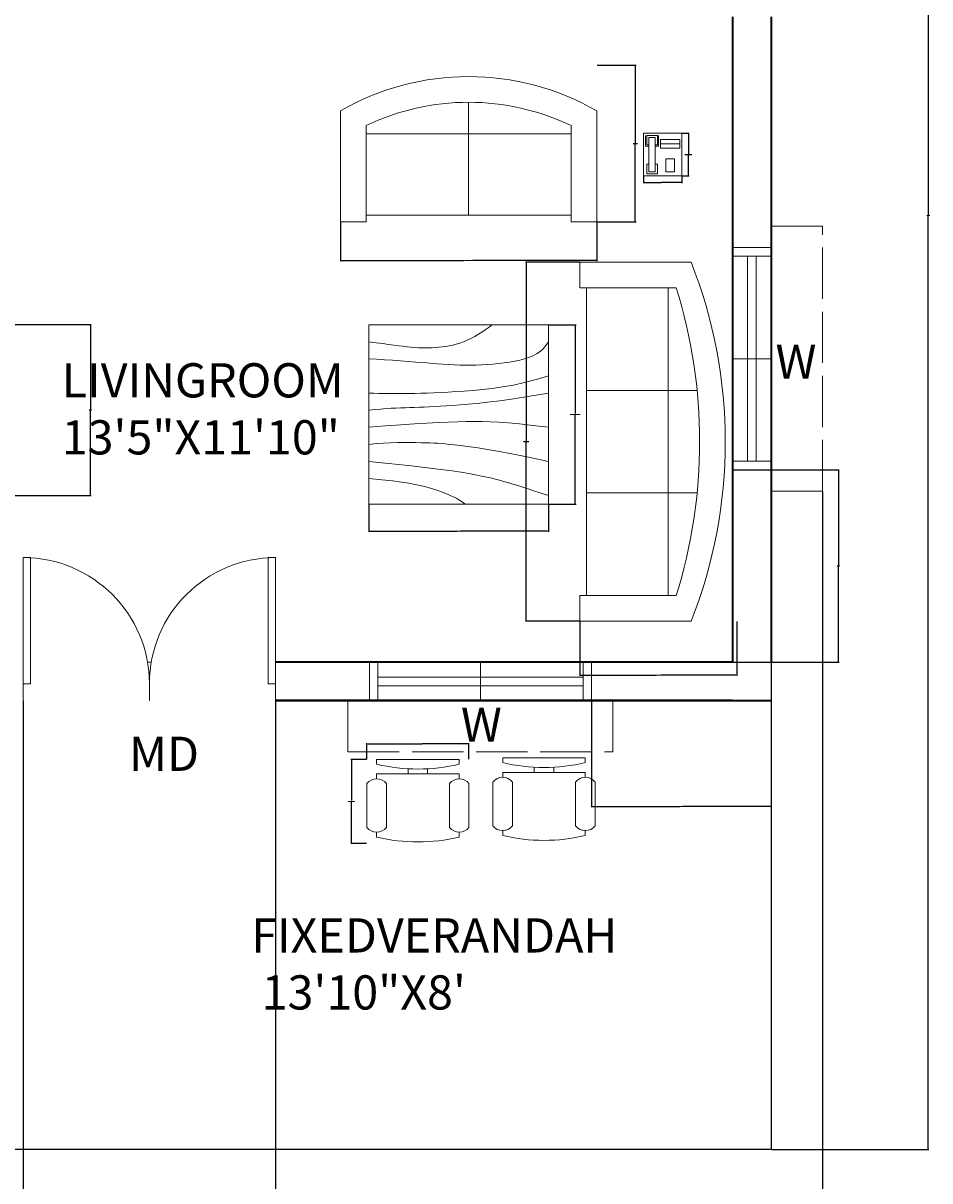
# Model space of a CAD drawing. Units: inches. Extents: x -35 to 832, y -515 to 219.
# Tile 4 of 7: x 179 to 391, y -262 to 9. Entities that reach past the tile are written whole.
import ezdxf

# ---------------------------------------------------------------- set-up
doc = ezdxf.new("R2010")
doc.units = ezdxf.units.IN
doc.header["$MEASUREMENT"] = 0
doc.linetypes.add('ACAD_ISO02W100', pattern=[15, 12, -3])
for name, color, linetype, lineweight in [('A-ANNO-TEXT', 7, 'Continuous', 18), ('A-AREA-IDEN', 7, 'Continuous', 18), ('A-DOOR', 4, 'Continuous', 18), ('A-EQPM', 8, 'Continuous', 18), ('A-FLOR', 7, 'Continuous', 25), ('A-FURN', 8, 'Continuous', 18), ('A-GLAZ', 2, 'Continuous', 18), ('A-GLAZ-OVHD', 2, 'ACAD_ISO02W100', 13), ('A-WALL', 10, 'Continuous', 35), ('S-ANNO-DIMS', 2, 'Continuous', 18)]:
    doc.layers.add(name, color=color, linetype=linetype, lineweight=lineweight)
doc.styles.get("Standard").update_dxf_attribs({"font": 'arial.ttf'})
doc.dimstyles.get("Standard").update_dxf_attribs({"dimtxt": 0.18, "dimasz": 0.18, "dimexe": 0.18, "dimexo": 0.0625, "dimgap": 0.09, "dimtad": 0, "dimtih": 1, "dimtoh": 1, "dimdec": 1, "dimzin": 0, "dimdsep": 46, "dimlunit": 4, "dimtxsty": 'Standard', "dimcen": 0.09, "dimclrd": 211, "dimclre": 4, "dimclrt": 3, "dimadec": 0, "dimazin": 0, "dimtfac": 0.5, "dimtdec": 1, "dimtofl": 0, "dimtmove": 0, "dimatfit": 3, "dimfxl": 1, "dimtfill": 2, "dimtfillclr": 61, "dimtolj": 1, "dimtzin": 0, "dimarcsym": 0})

# ---------------------------------------------------------------- blocks, each defined once
blk = doc.blocks.new('Chair - Desk')
for p, q in [((-8.5, 0), (-8.5, -1)), ((-8.5, 0), (8.5, 0)), ((8.5, 0), (8.5, -1)), ((-2, -3), (-2, -1.9355)), ((2, -1.9576), (2, -3)), ((-8.5, -3), (-8.5, -4)), ((-8.5, -3), (8.5, -3)), ((8.5, -3), (8.5, -4)), ((-10.5, -5), (-10.5, -14)), ((-6.5, -14), (-6.5, -5)), ((6.5, -5), (6.5, -14)), ((10.5, -14), (10.5, -5)), ((-8.5, -15), (-8.5, -16)), ((8.5, -15), (8.5, -16))]:
    blk.add_line(p, q)
for centre, radius, start, end in [((0, 34.625), 36.625, 256.5803, 283.4197), ((-8.5, -6.5), 2.5, 36.8699, 143.1301), ((8.5, -6.5), 2.5, 36.8699, 143.1301), ((-8.5, -12.5), 2.5, 216.8699, 323.1301), ((8.5, -12.5), 2.5, 216.8699, 323.1301), ((0, 19.625), 36.625, 256.5803, 283.4197)]:
    blk.add_arc(centre, radius, start, end)
blk = doc.blocks.new('Table - Square Woodgrain 42 x 42 in.')
blk.add_line((0, -42), (42, -42))
for points in [[(0, -4), (1.704, -4.2172), (3.2358, -4.4188), (4.615, -4.604), (5.8615, -4.7721), (6.9951, -4.9224), (8.0357, -5.0541), (9.0031, -5.1667), (9.9171, -5.2594), (10.7951, -5.3316), (11.6445, -5.3836), (12.4702, -5.4157), (13.277, -5.4283), (14.0698, -5.4217), (14.8535, -5.3964), (15.6331, -5.3526), (16.4133, -5.2908), (17.1986, -5.2103), (17.9913, -5.1062), (18.793, -4.9727), (19.6056, -4.8038), (20.4307, -4.5937), (21.2701, -4.3365), (22.1256, -4.0262), (22.9989, -3.6571), (23.888, -3.2272), (24.7756, -2.7516), (25.6408, -2.2491), (26.4624, -1.7387), (27.2195, -1.2395), (27.891, -0.7703), (28.456, -0.3501), (28.8934, 0.002)], [(0, -42), (0, 0), (42, 0), (42, -42)], [(0, -8), (1.8203, -8.1001), (3.6741, -8.2149), (5.5411, -8.3408), (7.4011, -8.4741), (9.2339, -8.6112), (11.0193, -8.7484), (12.7371, -8.8821), (14.3671, -9.0086), (15.8954, -9.1246), (17.3337, -9.2278), (18.6997, -9.3159), (20.0116, -9.387), (21.2871, -9.4389), (22.5442, -9.4696), (23.8008, -9.477), (25.0749, -9.459), (26.3791, -9.4137), (27.7049, -9.3403), (29.0383, -9.2382), (30.3655, -9.1068), (31.6728, -8.9455), (32.9461, -8.7535), (34.1717, -8.5304), (35.3358, -8.2756), (36.4268, -7.9863), (37.443, -7.6521), (38.3849, -7.2603), (39.253, -6.7986), (40.048, -6.2542), (40.7705, -5.6147), (41.421, -4.8674), (42, -4)], [(42, -12), (39.1784, -12.8621), (36.4519, -13.5654), (33.8246, -14.1294), (31.3004, -14.5731), (28.8832, -14.9161), (26.577, -15.1775), (24.3858, -15.3768), (22.3136, -15.5332), (20.3622, -15.6632), (18.5254, -15.7718), (16.7947, -15.8612), (15.1618, -15.9338), (13.6183, -15.9916), (12.1558, -16.0369), (10.7659, -16.0718), (9.4403, -16.0987), (8.1703, -16.1191), (6.9461, -16.1325), (5.7577, -16.1377), (4.595, -16.1335), (3.4479, -16.1188), (2.3064, -16.0924), (1.1604, -16.0532), (0, -16)], [(42, -16), (37.6529, -16.7365), (33.8802, -17.329), (30.6179, -17.7961), (27.8015, -18.1561), (25.3668, -18.4275), (23.2497, -18.6288), (21.3859, -18.7785), (19.7111, -18.8949), (18.1693, -18.9939), (16.7375, -19.0795), (15.401, -19.1534), (14.1449, -19.217), (12.9544, -19.2717), (11.8148, -19.3191), (10.7113, -19.3606), (9.6291, -19.3976), (8.5534, -19.4323), (7.47, -19.4689), (6.3643, -19.5122), (5.222, -19.5672), (4.0288, -19.6386), (2.7703, -19.7313), (1.4321, -19.8501), (0, -20)], [(0, -24), (3.9243, -23.6805), (7.4766, -23.4138), (10.6891, -23.1954), (13.5943, -23.0205), (16.2247, -22.8847), (18.6125, -22.7832), (20.7903, -22.7116), (22.7903, -22.6651), (24.6563, -22.642), (26.4764, -22.6507), (28.35, -22.7024), (30.3766, -22.8084), (32.6555, -22.98), (35.2861, -23.2283), (38.3678, -23.5645), (42, -24)], [(42, -32), (37.392, -31.017), (33.4585, -30.2231), (30.1291, -29.5949), (27.3334, -29.109), (25.0009, -28.742), (23.0612, -28.4707), (21.4439, -28.2716), (20.0786, -28.1215), (18.8998, -28.0002), (17.8609, -27.9014), (16.9206, -27.8219), (16.0371, -27.7588), (15.1691, -27.709), (14.2748, -27.6693), (13.3128, -27.6368), (12.2415, -27.6083), (11.0295, -27.5824), (9.6867, -27.5643), (8.233, -27.5608), (6.6884, -27.5787), (5.0728, -27.6248), (3.4062, -27.7058), (1.7086, -27.8286), (0, -28)], [(0, -32), (5.4026, -32.5358), (9.9494, -33.019), (13.7424, -33.4553), (16.8834, -33.8505), (19.4743, -34.2106), (21.6171, -34.5413), (23.4136, -34.8486), (24.9657, -35.1382), (26.3614, -35.4156), (27.6332, -35.6841), (28.7995, -35.9467), (29.8788, -36.2064), (30.8897, -36.4661), (31.8507, -36.7288), (32.7802, -36.9973), (33.6968, -37.2747), (34.6175, -37.5635), (35.5531, -37.8651), (36.5128, -38.1805), (37.506, -38.5108), (38.5421, -38.8568), (39.6302, -39.2197), (40.7797, -39.6004), (42, -40)], [(0, -36), (3.0098, -36.2857), (5.5354, -36.5643), (7.6368, -36.8359), (9.374, -37.1009), (10.807, -37.3597), (11.9957, -37.6126), (13.0002, -37.8599), (13.8804, -38.102), (14.6874, -38.3393), (15.4365, -38.5729), (16.1338, -38.8041), (16.7858, -39.0341), (17.3987, -39.264), (17.9787, -39.4952), (18.5322, -39.7288), (19.0655, -39.9662), (19.5832, -40.2081), (20.0842, -40.4544), (20.5657, -40.7046), (21.0249, -40.9581), (21.459, -41.2144), (21.8653, -41.4731), (22.2409, -41.7335), (22.5831, -41.9951)]]:
    blk.add_lwpolyline(points)
blk = doc.blocks.new('Sofa - Roundback 7 ft.')
for p, q in [((-12.00002, -32.4421), (-12.00003, -6.5971)), ((11.99997, -32.4421), (11.99998, -6.5971)), ((-36.000027, -34), (-36.000027, -11.4696)), ((-35.999844, -13.3819), (35.9998, -13.3819)), ((35.99998, -34), (35.99998, -11.4696)), ((-36.000027, -32.4421), (35.99998, -32.4421))]:
    blk.add_line(p, q)
for points in [[(-36.000027, -34), (-42.000027, -34), (-42.000027, -8)], [(41.99998, -8), (41.99998, -34), (35.99998, -34)]]:
    blk.add_lwpolyline(points)
for centre, radius, start, end in [((0, -114.25), 114.25, 68.43141, 111.5686), ((-0.00001, -127.1968), 121.1968, 72.72033, 107.2797)]:
    blk.add_arc(centre, radius, start, end)
blk = doc.blocks.new('Sofa - Roundback Loveseat 5 ft.')
for p, q in [((0, -32.44198), (0, -5.99998)), ((-24, -33.99998), (-24, -11.46958)), ((-23.9998, -13.38178), (23.99986, -13.38178)), ((24.00004, -33.99998), (24.00004, -11.46958)), ((-24, -32.44198), (24.00004, -32.44198))]:
    blk.add_line(p, q)
for points in [[(-24, -33.99998), (-30, -33.99998), (-30, -7.99998)], [(30.00004, -7.99998), (30.00004, -33.99998), (24.00004, -33.99998)]]:
    blk.add_lwpolyline(points)
for centre, radius, start, end in [((0, -60.24998), 60.24998, 60.13715, 119.8628), ((0, -61.38438), 55.38444, 64.32083, 115.6792)]:
    blk.add_arc(centre, radius, start, end)
blk = doc.blocks.new('Phone - Desk')
for p, q in [((-4.5, -5), (-4.5, 5)), ((-4.5, 5), (4.5, 5)), ((-4, 4.5), (-4, 2)), ((-3.75, 4.5), (-3.75, 2.25)), ((-1.25, 4.5), (-3.75, 4.5)), ((-3.25, 4), (-3.25, -4)), ((-3.25, 4), (-1.75, 4)), ((-1.75, -4), (-1.75, 4)), ((-1.25, 2.25), (-1.25, 4.5)), ((-1, 2), (-1, 4.5)), ((4, 3.5), (-0.5, 3.5)), ((-0.5, 3.5), (-0.5, 1.5)), ((4, 1.5), (4, 3.5)), ((4.5, 5), (4.5, -5)), ((-4, 2), (-3.25, 2)), ((-3.75, 2.25), (-3.25, 2.25)), ((-1.75, 2.25), (-1.25, 2.25)), ((-1.75, 2), (-1, 2)), ((-0.5, 2.5), (4, 2.5)), ((-0.5, 1.5), (4, 1.5)), ((-3.75, -2.25), (-3.25, -2.25)), ((-3.75, -4.5), (-3.75, -2.25)), ((-1.75, -2.25), (-1.25, -2.25)), ((-1.25, -2.25), (-1.25, -4.5)), ((2.75, -1), (0.75, -1)), ((0.75, -1), (0.75, -4)), ((2.75, -4), (2.75, -1)), ((4.5, -5), (-4.5, -5)), ((-1.25, -4.5), (-3.75, -4.5)), ((-3.25, -4), (-1.75, -4)), ((0.75, -4), (2.75, -4))]:
    blk.add_line(p, q)
blk = doc.blocks.new('*U4')
for p, q in [((0, 0), (0, -100)), ((750, 0), (750, -100))]:
    blk.add_line(p, q)
blk.add_lwpolyline([(0, 0), (0, 750), (43.75, 750), (43.75, 0)], close=True)
blk.add_arc((0, 0), 750, 0, 90)
blk = doc.blocks.new('WIN-48')
for p, q in [((0, 9), (0, 0)), ((2, 9), (2, 0)), ((26, 9), (26, 0)), ((50, 9), (50, 0)), ((52, 9), (52, 0)), ((2, 5.5), (50, 5.5)), ((2, 3.5), (50, 3.5))]:
    blk.add_line(p, q)
blk = doc.blocks.new('WIN-48-HOOD')
for p, q in [((5, 12), (0, 12)), ((0, 12), (0, 0)), ((57, 12), (62, 12)), ((62, 12), (62, 0)), ((0, 0), (62, 0))]:
    blk.add_line(p, q)
blk = doc.blocks.new('*D71')
at = {"layer": 'Defpoints', "color": 0, "transparency": 16777216}
for p in [(283.1, -160.09), (259.23, -163.68), (283.1, -163.68)]:
    blk.add_point(p, dxfattribs=at)
at = {"layer": 'S-ANNO-DIMS', "color": 4, "lineweight": -2, "transparency": 16777216}
for p, q in [((259.23, -163.61), (259.23, -159.91)), ((283.1, -163.61), (283.1, -159.91))]:
    blk.add_line(p, q, dxfattribs=at)
at = {"layer": 'S-ANNO-DIMS', "color": 211, "lineweight": -2, "transparency": 16777216}
for p, q in [((259.41, -160.09), (270.1, -160.09)), ((282.92, -160.09), (272.23, -160.09))]:
    blk.add_line(p, q, dxfattribs=at)
at = {"layer": 'S-ANNO-DIMS', "color": 211, "transparency": 16777216}
for points in [[(259.41, -160.06), (259.41, -160.12), (259.23, -160.09)], [(282.92, -160.06), (282.92, -160.12), (283.1, -160.09)]]:
    blk.add_solid(points, dxfattribs=at)
at = {"layer": 'S-ANNO-DIMS', "color": 3, "transparency": 16777216, "insert": (271.17, -160.09), "char_height": 0.18, "attachment_point": 5, "bg_fill": 1, "box_fill_scale": 1.25, "bg_fill_color": 61, "bg_fill_transparency": 0}
blk.add_mtext('\\A1;CHAIR 2\'-0" TYP.', dxfattribs=at)
blk = doc.blocks.new('*D72')
at = {"layer": 'Defpoints', "color": 0, "transparency": 16777216}
for p in [(255.65, -163.68), (259.23, -163.68), (259.23, -183.38)]:
    blk.add_point(p, dxfattribs=at)
at = {"layer": 'S-ANNO-DIMS', "color": 4, "lineweight": -2, "transparency": 16777216}
for p, q in [((259.17, -163.68), (255.47, -163.68)), ((259.17, -183.38), (255.47, -183.38))]:
    blk.add_line(p, q, dxfattribs=at)
at = {"layer": 'S-ANNO-DIMS', "color": 211, "lineweight": -2, "transparency": 16777216}
for p, q in [((255.65, -163.86), (255.65, -173.34)), ((255.65, -183.2), (255.65, -173.71))]:
    blk.add_line(p, q, dxfattribs=at)
at = {"layer": 'S-ANNO-DIMS', "color": 211, "transparency": 16777216}
for points in [[(255.62, -163.86), (255.68, -163.86), (255.65, -163.68)], [(255.62, -183.2), (255.68, -183.2), (255.65, -183.38)]]:
    blk.add_solid(points, dxfattribs=at)
at = {"layer": 'S-ANNO-DIMS', "color": 3, "transparency": 16777216, "insert": (255.65, -173.53), "char_height": 0.18, "attachment_point": 5, "bg_fill": 1, "box_fill_scale": 1.25, "bg_fill_color": 61, "bg_fill_transparency": 0}
blk.add_mtext('\\A1;1\'-7 1/2" TYP.', dxfattribs=at)
blk = doc.blocks.new('*D95')
at = {"layer": 'Defpoints', "color": 0, "transparency": 16777216}
for p in [(301.68, -61.99), (307.98, -61.99), (301.68, -103.99)]:
    blk.add_point(p, dxfattribs=at)
at = {"layer": 'S-ANNO-DIMS', "color": 4, "lineweight": -2, "transparency": 16777216}
for p, q in [((301.74, -61.99), (308.16, -61.99)), ((301.74, -103.99), (308.16, -103.99))]:
    blk.add_line(p, q, dxfattribs=at)
at = {"layer": 'S-ANNO-DIMS', "color": 211, "lineweight": -2, "transparency": 16777216}
for p, q in [((307.98, -62.17), (307.98, -82.81)), ((307.98, -103.81), (307.98, -83.18))]:
    blk.add_line(p, q, dxfattribs=at)
at = {"layer": 'S-ANNO-DIMS', "color": 211, "transparency": 16777216}
for points in [[(307.95, -62.17), (308.01, -62.17), (307.98, -61.99)], [(307.95, -103.81), (308.01, -103.81), (307.98, -103.99)]]:
    blk.add_solid(points, dxfattribs=at)
at = {"layer": 'S-ANNO-DIMS', "color": 3, "transparency": 16777216, "insert": (307.98, -82.99), "char_height": 0.18, "attachment_point": 5, "bg_fill": 1, "box_fill_scale": 1.25, "bg_fill_color": 61, "bg_fill_transparency": 0}
blk.add_mtext('\\A1;COFFEE TABLE 3\'-6"', dxfattribs=at)
blk = doc.blocks.new('*D96')
at = {"layer": 'Defpoints', "color": 0, "transparency": 16777216}
for p in [(259.68, -103.99), (301.68, -103.99), (301.68, -110.29)]:
    blk.add_point(p, dxfattribs=at)
at = {"layer": 'S-ANNO-DIMS', "color": 4, "lineweight": -2, "transparency": 16777216}
for p, q in [((259.68, -104.06), (259.68, -110.47)), ((301.68, -104.06), (301.68, -110.47))]:
    blk.add_line(p, q, dxfattribs=at)
at = {"layer": 'S-ANNO-DIMS', "color": 211, "lineweight": -2, "transparency": 16777216}
for p, q in [((259.86, -110.29), (280.35, -110.29)), ((301.5, -110.29), (281.01, -110.29))]:
    blk.add_line(p, q, dxfattribs=at)
at = {"layer": 'S-ANNO-DIMS', "color": 211, "transparency": 16777216}
for points in [[(259.86, -110.26), (259.86, -110.32), (259.68, -110.29)], [(301.5, -110.26), (301.5, -110.32), (301.68, -110.29)]]:
    blk.add_solid(points, dxfattribs=at)
at = {"layer": 'S-ANNO-DIMS', "color": 3, "transparency": 16777216, "insert": (280.68, -110.29), "char_height": 0.18, "attachment_point": 5, "bg_fill": 1, "box_fill_scale": 1.25, "bg_fill_color": 61, "bg_fill_transparency": 0}
blk.add_mtext('\\A1;3\'-6"', dxfattribs=at)
blk = doc.blocks.new('*D97')
at = {"layer": 'Defpoints', "color": 0, "transparency": 16777216}
for p in [(309.08, -47.37), (296.48, -131.37), (309.08, -131.37)]:
    blk.add_point(p, dxfattribs=at)
at = {"layer": 'S-ANNO-DIMS', "color": 4, "lineweight": -2, "transparency": 16777216}
for p, q in [((309.02, -47.37), (296.3, -47.37)), ((309.02, -131.37), (296.3, -131.37))]:
    blk.add_line(p, q, dxfattribs=at)
at = {"layer": 'S-ANNO-DIMS', "color": 211, "lineweight": -2, "transparency": 16777216}
for p, q in [((296.48, -47.55), (296.48, -89.19)), ((296.48, -131.19), (296.48, -89.55))]:
    blk.add_line(p, q, dxfattribs=at)
at = {"layer": 'S-ANNO-DIMS', "color": 211, "transparency": 16777216}
for points in [[(296.45, -47.55), (296.51, -47.55), (296.48, -47.37)], [(296.45, -131.19), (296.51, -131.19), (296.48, -131.37)]]:
    blk.add_solid(points, dxfattribs=at)
at = {"layer": 'S-ANNO-DIMS', "color": 3, "transparency": 16777216, "insert": (296.48, -89.37), "char_height": 0.18, "attachment_point": 5, "bg_fill": 1, "box_fill_scale": 1.25, "bg_fill_color": 61, "bg_fill_transparency": 0}
blk.add_mtext('\\A1;SOFA 7\'-0"', dxfattribs=at)
blk = doc.blocks.new('*D98')
at = {"layer": 'Defpoints', "color": 0, "transparency": 16777216}
for p in [(309.08, -131.37), (345.75, -131.37), (345.75, -143.97)]:
    blk.add_point(p, dxfattribs=at)
at = {"layer": 'S-ANNO-DIMS', "color": 4, "lineweight": -2, "transparency": 16777216}
for p, q in [((309.08, -131.43), (309.08, -144.15)), ((345.75, -131.43), (345.75, -144.15))]:
    blk.add_line(p, q, dxfattribs=at)
at = {"layer": 'S-ANNO-DIMS', "color": 211, "lineweight": -2, "transparency": 16777216}
for p, q in [((309.26, -143.97), (326.88, -143.97)), ((345.57, -143.97), (327.96, -143.97))]:
    blk.add_line(p, q, dxfattribs=at)
at = {"layer": 'S-ANNO-DIMS', "color": 211, "transparency": 16777216}
for points in [[(309.26, -143.94), (309.26, -144), (309.08, -143.97)], [(345.57, -143.94), (345.57, -144), (345.75, -143.97)]]:
    blk.add_solid(points, dxfattribs=at)
at = {"layer": 'S-ANNO-DIMS', "color": 3, "transparency": 16777216, "insert": (327.42, -143.97), "char_height": 0.18, "attachment_point": 5, "bg_fill": 1, "box_fill_scale": 1.25, "bg_fill_color": 61, "bg_fill_transparency": 0}
blk.add_mtext('\\A1;3\'-0 1/2"', dxfattribs=at)
blk = doc.blocks.new('*D99')
at = {"layer": 'Defpoints', "color": 0, "transparency": 16777216}
for p in [(253.02, -37.96), (313.02, -37.96), (313.02, -46.96)]:
    blk.add_point(p, dxfattribs=at)
at = {"layer": 'S-ANNO-DIMS', "color": 4, "lineweight": -2, "transparency": 16777216}
for p, q in [((253.02, -38.03), (253.02, -47.14)), ((313.02, -38.03), (313.02, -47.14))]:
    blk.add_line(p, q, dxfattribs=at)
at = {"layer": 'S-ANNO-DIMS', "color": 211, "lineweight": -2, "transparency": 16777216}
for p, q in [((253.2, -46.96), (281.99, -46.96)), ((312.84, -46.96), (284.04, -46.96))]:
    blk.add_line(p, q, dxfattribs=at)
at = {"layer": 'S-ANNO-DIMS', "color": 211, "transparency": 16777216}
for points in [[(253.2, -46.93), (253.2, -46.99), (253.02, -46.96)], [(312.84, -46.93), (312.84, -46.99), (313.02, -46.96)]]:
    blk.add_solid(points, dxfattribs=at)
at = {"layer": 'S-ANNO-DIMS', "color": 3, "transparency": 16777216, "insert": (283.02, -46.96), "char_height": 0.18, "attachment_point": 5, "bg_fill": 1, "box_fill_scale": 1.25, "bg_fill_color": 61, "bg_fill_transparency": 0}
blk.add_mtext('\\A1;LOVESEAT 5\'-0"', dxfattribs=at)
blk = doc.blocks.new('*D100')
at = {"layer": 'Defpoints', "color": 0, "transparency": 16777216}
for p in [(313.02, -1.3), (322.02, -1.3), (313.02, -37.96)]:
    blk.add_point(p, dxfattribs=at)
at = {"layer": 'S-ANNO-DIMS', "color": 4, "lineweight": -2, "transparency": 16777216}
for p, q in [((313.08, -1.3), (322.2, -1.3)), ((313.08, -37.96), (322.2, -37.96))]:
    blk.add_line(p, q, dxfattribs=at)
at = {"layer": 'S-ANNO-DIMS', "color": 211, "lineweight": -2, "transparency": 16777216}
for p, q in [((322.02, -1.48), (322.02, -19.45)), ((322.02, -37.78), (322.02, -19.81))]:
    blk.add_line(p, q, dxfattribs=at)
at = {"layer": 'S-ANNO-DIMS', "color": 211, "transparency": 16777216}
for points in [[(321.99, -1.48), (322.05, -1.48), (322.02, -1.3)], [(321.99, -37.78), (322.05, -37.78), (322.02, -37.96)]]:
    blk.add_solid(points, dxfattribs=at)
at = {"layer": 'S-ANNO-DIMS', "color": 3, "transparency": 16777216, "insert": (322.02, -19.63), "char_height": 0.18, "attachment_point": 5, "bg_fill": 1, "box_fill_scale": 1.25, "bg_fill_color": 61, "bg_fill_transparency": 0}
blk.add_mtext('\\A1;3\'-0 1/2"', dxfattribs=at)
blk = doc.blocks.new('*D101')
at = {"layer": 'Defpoints', "color": 0, "transparency": 16777216}
for p in [(332.94, -17.2), (334.44, -17.2), (332.94, -27.2)]:
    blk.add_point(p, dxfattribs=at)
at = {"layer": 'S-ANNO-DIMS', "color": 4, "lineweight": -2, "transparency": 16777216}
for p, q in [((333, -17.2), (334.62, -17.2)), ((333, -27.2), (334.62, -27.2))]:
    blk.add_line(p, q, dxfattribs=at)
at = {"layer": 'S-ANNO-DIMS', "color": 211, "lineweight": -2, "transparency": 16777216}
for p, q in [((334.44, -17.38), (334.44, -22.02)), ((334.44, -27.02), (334.44, -22.38))]:
    blk.add_line(p, q, dxfattribs=at)
at = {"layer": 'S-ANNO-DIMS', "color": 211, "transparency": 16777216}
for points in [[(334.41, -17.38), (334.47, -17.38), (334.44, -17.2)], [(334.41, -27.02), (334.47, -27.02), (334.44, -27.2)]]:
    blk.add_solid(points, dxfattribs=at)
at = {"layer": 'S-ANNO-DIMS', "color": 3, "transparency": 16777216, "insert": (334.44, -22.2), "char_height": 0.18, "attachment_point": 5, "bg_fill": 1, "box_fill_scale": 1.25, "bg_fill_color": 61, "bg_fill_transparency": 0}
blk.add_mtext('\\A1;PHONE 0\'-10"', dxfattribs=at)
blk = doc.blocks.new('*D102')
at = {"layer": 'Defpoints', "color": 0, "transparency": 16777216}
for p in [(323.94, -27.2), (332.94, -27.2), (332.94, -28.7)]:
    blk.add_point(p, dxfattribs=at)
at = {"layer": 'S-ANNO-DIMS', "color": 4, "lineweight": -2, "transparency": 16777216}
for p, q in [((323.94, -27.26), (323.94, -28.88)), ((332.94, -27.26), (332.94, -28.88))]:
    blk.add_line(p, q, dxfattribs=at)
at = {"layer": 'S-ANNO-DIMS', "color": 211, "lineweight": -2, "transparency": 16777216}
for p, q in [((324.12, -28.7), (328.11, -28.7)), ((332.76, -28.7), (328.77, -28.7))]:
    blk.add_line(p, q, dxfattribs=at)
at = {"layer": 'S-ANNO-DIMS', "color": 211, "transparency": 16777216}
for points in [[(324.12, -28.67), (324.12, -28.73), (323.94, -28.7)], [(332.76, -28.67), (332.76, -28.73), (332.94, -28.7)]]:
    blk.add_solid(points, dxfattribs=at)
at = {"layer": 'S-ANNO-DIMS', "color": 3, "transparency": 16777216, "insert": (328.44, -28.7), "char_height": 0.18, "attachment_point": 5, "bg_fill": 1, "box_fill_scale": 1.25, "bg_fill_color": 61, "bg_fill_transparency": 0}
blk.add_mtext('\\A1;0\'-9"', dxfattribs=at)
blk = doc.blocks.new('*D106')
at = {"layer": 'Defpoints', "color": 0, "transparency": 16777216}
for p in [(353.8, 182.05), (353.8, -254.95), (390.55, -254.95)]:
    blk.add_point(p, dxfattribs=at)
at = {"layer": 'S-ANNO-DIMS', "color": 4, "lineweight": -2, "transparency": 16777216}
for p, q in [((353.86, 182.05), (390.73, 182.05)), ((353.86, -254.95), (390.73, -254.95))]:
    blk.add_line(p, q, dxfattribs=at)
at = {"layer": 'S-ANNO-DIMS', "color": 211, "lineweight": -2, "transparency": 16777216}
for p, q in [((390.55, 181.87), (390.55, -36.27)), ((390.55, -254.77), (390.55, -36.63))]:
    blk.add_line(p, q, dxfattribs=at)
at = {"layer": 'S-ANNO-DIMS', "color": 211, "transparency": 16777216}
for points in [[(390.52, 181.87), (390.58, 181.87), (390.55, 182.05)], [(390.52, -254.77), (390.58, -254.77), (390.55, -254.95)]]:
    blk.add_solid(points, dxfattribs=at)
at = {"layer": 'S-ANNO-DIMS', "color": 3, "transparency": 16777216, "insert": (390.55, -36.45), "char_height": 0.18, "attachment_point": 5, "bg_fill": 1, "box_fill_scale": 1.25, "bg_fill_color": 61, "bg_fill_transparency": 0}
blk.add_mtext('\\A1;36\'-5"', dxfattribs=at)
blk = doc.blocks.new('*D109')
at = {"layer": 'Defpoints', "color": 0, "transparency": 16777216}
for p in [(365.8, -100.95), (-10.2, -143.45), (365.8, -279.7)]:
    blk.add_point(p, dxfattribs=at)
at = {"layer": 'S-ANNO-DIMS', "color": 4, "lineweight": -2, "transparency": 16777216}
for p, q in [((365.8, -101.01), (365.8, -279.88)), ((-10.2, -143.51), (-10.2, -279.88))]:
    blk.add_line(p, q, dxfattribs=at)
at = {"layer": 'S-ANNO-DIMS', "color": 211, "lineweight": -2, "transparency": 16777216}
for p, q in [((-10.02, -279.7), (177.4, -279.7)), ((365.62, -279.7), (178.2, -279.7))]:
    blk.add_line(p, q, dxfattribs=at)
at = {"layer": 'S-ANNO-DIMS', "color": 211, "transparency": 16777216}
for points in [[(-10.02, -279.67), (-10.02, -279.73), (-10.2, -279.7)], [(365.62, -279.67), (365.62, -279.73), (365.8, -279.7)]]:
    blk.add_solid(points, dxfattribs=at)
at = {"layer": 'S-ANNO-DIMS', "color": 3, "transparency": 16777216, "insert": (177.8, -279.7), "char_height": 0.18, "attachment_point": 5, "bg_fill": 1, "box_fill_scale": 1.25, "bg_fill_color": 61, "bg_fill_transparency": 0}
blk.add_mtext('\\A1;31\'-4"', dxfattribs=at)
blk = doc.blocks.new('*D111')
at = {"layer": 'Defpoints', "color": 0, "transparency": 16777216}
for p in [(178.8, -149.95), (237.86, -149.95), (237.86, -279.7)]:
    blk.add_point(p, dxfattribs=at)
at = {"layer": 'S-ANNO-DIMS', "color": 4, "lineweight": -2, "transparency": 16777216}
for p, q in [((178.8, -150.01), (178.8, -279.88)), ((237.86, -150.01), (237.86, -279.88))]:
    blk.add_line(p, q, dxfattribs=at)
at = {"layer": 'S-ANNO-DIMS', "color": 211, "lineweight": -2, "transparency": 16777216}
for p, q in [((178.98, -279.7), (207.93, -279.7)), ((237.68, -279.7), (208.73, -279.7))]:
    blk.add_line(p, q, dxfattribs=at)
at = {"layer": 'S-ANNO-DIMS', "color": 211, "transparency": 16777216}
for points in [[(178.98, -279.67), (178.98, -279.73), (178.8, -279.7)], [(237.68, -279.67), (237.68, -279.73), (237.86, -279.7)]]:
    blk.add_solid(points, dxfattribs=at)
at = {"layer": 'S-ANNO-DIMS', "color": 3, "transparency": 16777216, "insert": (208.33, -279.7), "char_height": 0.18, "attachment_point": 5, "bg_fill": 1, "box_fill_scale": 1.25, "bg_fill_color": 61, "bg_fill_transparency": 0}
blk.add_mtext('\\A1;4\'-11"', dxfattribs=at)
blk = doc.blocks.new('*D114')
at = {"layer": 'Defpoints', "color": 0, "transparency": 16777216}
for p in [(169.8, -61.95), (169.8, -101.95), (194.55, -101.95)]:
    blk.add_point(p, dxfattribs=at)
at = {"layer": 'S-ANNO-DIMS', "color": 4, "lineweight": -2, "transparency": 16777216}
for p, q in [((169.86, -61.95), (194.73, -61.95)), ((169.86, -101.95), (194.73, -101.95))]:
    blk.add_line(p, q, dxfattribs=at)
at = {"layer": 'S-ANNO-DIMS', "color": 211, "lineweight": -2, "transparency": 16777216}
for p, q in [((194.55, -62.13), (194.55, -81.77)), ((194.55, -101.77), (194.55, -82.13))]:
    blk.add_line(p, q, dxfattribs=at)
at = {"layer": 'S-ANNO-DIMS', "color": 211, "transparency": 16777216}
for points in [[(194.52, -62.13), (194.58, -62.13), (194.55, -61.95)], [(194.52, -101.77), (194.58, -101.77), (194.55, -101.95)]]:
    blk.add_solid(points, dxfattribs=at)
at = {"layer": 'S-ANNO-DIMS', "color": 3, "transparency": 16777216, "insert": (194.55, -81.95), "char_height": 0.18, "attachment_point": 5, "bg_fill": 1, "box_fill_scale": 1.25, "bg_fill_color": 61, "bg_fill_transparency": 0}
blk.add_mtext('\\A1;3\'-4"', dxfattribs=at)
blk = doc.blocks.new('*D120')
at = {"layer": 'Defpoints', "color": 0, "transparency": 16777216}
for p in [(344.8, -95.95), (344.8, -140.95), (369.55, -140.95)]:
    blk.add_point(p, dxfattribs=at)
at = {"layer": 'S-ANNO-DIMS', "color": 4, "lineweight": -2, "transparency": 16777216}
for p, q in [((344.86, -95.95), (369.73, -95.95)), ((344.86, -140.95), (369.73, -140.95))]:
    blk.add_line(p, q, dxfattribs=at)
at = {"layer": 'S-ANNO-DIMS', "color": 211, "lineweight": -2, "transparency": 16777216}
for p, q in [((369.55, -96.13), (369.55, -118.27)), ((369.55, -140.77), (369.55, -118.63))]:
    blk.add_line(p, q, dxfattribs=at)
at = {"layer": 'S-ANNO-DIMS', "color": 211, "transparency": 16777216}
for points in [[(369.52, -96.13), (369.58, -96.13), (369.55, -95.95)], [(369.52, -140.77), (369.58, -140.77), (369.55, -140.95)]]:
    blk.add_solid(points, dxfattribs=at)
at = {"layer": 'S-ANNO-DIMS', "color": 3, "transparency": 16777216, "insert": (369.55, -118.45), "char_height": 0.18, "attachment_point": 5, "bg_fill": 1, "box_fill_scale": 1.25, "bg_fill_color": 61, "bg_fill_transparency": 0}
blk.add_mtext('\\A1;3\'-9"', dxfattribs=at)
blk = doc.blocks.new('*D121')
at = {"layer": 'Defpoints', "color": 0, "transparency": 16777216}
for p in [(311.8, -149.95), (353.8, -149.95), (311.8, -174.7)]:
    blk.add_point(p, dxfattribs=at)
at = {"layer": 'S-ANNO-DIMS', "color": 4, "lineweight": -2, "transparency": 16777216}
for p, q in [((311.8, -150.01), (311.8, -174.88)), ((353.8, -150.01), (353.8, -174.88))]:
    blk.add_line(p, q, dxfattribs=at)
at = {"layer": 'S-ANNO-DIMS', "color": 211, "lineweight": -2, "transparency": 16777216}
for p, q in [((311.98, -174.7), (332.47, -174.7)), ((353.62, -174.7), (333.13, -174.7))]:
    blk.add_line(p, q, dxfattribs=at)
at = {"layer": 'S-ANNO-DIMS', "color": 211, "transparency": 16777216}
for points in [[(311.98, -174.67), (311.98, -174.73), (311.8, -174.7)], [(353.62, -174.67), (353.62, -174.73), (353.8, -174.7)]]:
    blk.add_solid(points, dxfattribs=at)
at = {"layer": 'S-ANNO-DIMS', "color": 3, "transparency": 16777216, "insert": (332.8, -174.7), "char_height": 0.18, "attachment_point": 5, "bg_fill": 1, "box_fill_scale": 1.25, "bg_fill_color": 61, "bg_fill_transparency": 0}
blk.add_mtext('\\A1;3\'-6"', dxfattribs=at)

msp = doc.modelspace()

# ---------------------------------------------------------------- linework, layer by layer
at = {"layer": 'A-DOOR'}
msp.add_line((208.77, -140.95), (207.89, -140.95), dxfattribs=at)
at = {"layer": 'A-FLOR'}
for p, q in [((353.8, -61.95), (353.8, -254.95)), ((353.8, -254.95), (169.8, -254.95))]:
    msp.add_line(p, q, dxfattribs=at)
at = {"layer": 'A-WALL'}
for p, q in [((344.8, 10.05), (344.8, -140.95)), ((353.8, 10.05), (353.8, -140.95)), ((344.8, -140.95), (237.86, -140.95)), ((344.8, -149.95), (237.86, -149.95)), ((237.86, -149.95), (353.8, -149.95))]:
    msp.add_line(p, q, dxfattribs=at)

# ---------------------------------------------------------------- block references
at = {"layer": 'A-DOOR', "yscale": 0.0393700787401575, "zscale": 0.0393700787401575}
for p, xscale in [((178.8, -146.01), 0.0393700787401575), ((237.86, -146.01), -0.0393700787401575)]:
    msp.add_blockref('*U4', p, dxfattribs=dict(at, xscale=xscale))
at = {"layer": 'A-EQPM'}
msp.add_blockref('Phone - Desk', (328.44, -22.2), dxfattribs=at)
at = {"layer": 'A-FURN'}
for name, p in [('Sofa - Roundback Loveseat 5 ft.', (283.02, -3.96)), ('Table - Square Woodgrain 42 x 42 in.', (259.68, -61.99))]:
    msp.add_blockref(name, p, dxfattribs=at)
at = {"layer": 'A-FURN', "rotation": 270}
msp.add_blockref('Sofa - Roundback 7 ft.', (343.08, -89.37), dxfattribs=at)
at = {"layer": 'A-FURN', "xscale": 1.136842622745053, "yscale": 1.136842622745053, "zscale": 1.136842622745053}
for p in [(271.17, -163.68), (300.66, -163.31)]:
    msp.add_blockref('Chair - Desk', p, dxfattribs=at)
at = {"layer": 'A-GLAZ'}
for p, rotation in [((344.8, -43.95), 270.0000000000001), ((311.8, -140.95), 180)]:
    msp.add_blockref('WIN-48', p, dxfattribs=dict(at, rotation=rotation))
at = {"layer": 'A-GLAZ-OVHD', "rotation": 89.99999999999982}
msp.add_blockref('WIN-48-HOOD', (365.8, -100.95), dxfattribs=at)
at = {"layer": 'A-GLAZ-OVHD'}
msp.add_blockref('WIN-48-HOOD', (254.8, -161.95), dxfattribs=at)

# ---------------------------------------------------------------- texts
at = {"layer": 'A-ANNO-TEXT'}
for s, p in [('W', (354.83, -74.66)), ('W', (281.22, -159.58)), ('MD', (203.58, -166.38))]:
    msp.add_text(s, height=8, dxfattribs=at).set_placement(p)
at = {"layer": 'A-AREA-IDEN', "char_height": 8, "attachment_point": 1}
for s, insert in [('LIVINGROOM\\P13\'5"X11\'10"', (187.83, -71.01)), ('FIXEDVERANDAH\\P 13\'10"X8\'', (232.16, -200.87))]:
    msp.add_mtext_dynamic_manual_height_columns(s, width=50.3004, gutter_width=1, heights=[0], dxfattribs=dict(at, insert=insert))

# ---------------------------------------------------------------- dimensions: what is measured, and where the dimension line sits
at = {"layer": 'S-ANNO-DIMS'}
for base, p1, p2, angle, picture, middle in [((390.55, -254.95), (353.8, 182.05), (353.8, -254.95), 90, '*D106', (390.55, -36.45)), ((322.02, -1.3), (313.02, -37.96), (313.02, -1.3), 90, '*D100', (322.02, -19.63)), ((194.55, -101.95), (169.8, -61.95), (169.8, -101.95), 270, '*D114', (194.55, -81.95)), ((369.55, -140.95), (344.8, -95.95), (344.8, -140.95), 270, '*D120', (369.55, -118.45)), ((311.8, -174.7), (353.8, -149.95), (311.8, -149.95), 180, '*D121', (332.8, -174.7))]:
    dim = msp.add_linear_dim(base=base, p1=p1, p2=p2, angle=angle, dimstyle='Standard', override={"dimdec": 1, "dimlfac": 1, "dimrnd": 0, "dimzin": 1, "dimdsep": 46, "dimlunit": 4, "dimfrac": 2}, dxfattribs=at)
    dim.commit()
    dim.dimension.update_dxf_attribs({"geometry": picture, "text_midpoint": middle})
for base, p1, p2, angle, text, picture, middle in [((334.44, -17.2), (332.94, -27.2), (332.94, -17.2), 90, 'PHONE <>', '*D101', (334.44, -22.2)), ((296.48, -131.37), (309.08, -47.37), (309.08, -131.37), 270, 'SOFA <>', '*D97', (296.48, -89.37)), ((307.98, -61.99), (301.68, -103.99), (301.68, -61.99), 90, 'COFFEE TABLE <>', '*D95', (307.98, -82.99)), ((255.65, -163.68), (259.23, -183.38), (259.23, -163.68), 90, '<> TYP.', '*D72', (255.65, -173.53))]:
    dim = msp.add_linear_dim(base=base, p1=p1, p2=p2, angle=angle, text=text, dimstyle='Standard', override={"dimdec": 1, "dimlfac": 1, "dimrnd": 0, "dimzin": 1, "dimdsep": 46, "dimlunit": 4, "dimfrac": 2}, dxfattribs=at)
    dim.commit()
    dim.dimension.update_dxf_attribs({"geometry": picture, "text_midpoint": middle})
for base, p1, p2, picture, middle in [((332.94, -28.7), (323.94, -27.2), (332.94, -27.2), '*D102', (328.44, -28.7)), ((365.8, -279.7), (-10.2, -143.45), (365.8, -100.95), '*D109', (177.8, -279.7)), ((301.68, -110.29), (259.68, -103.99), (301.68, -103.99), '*D96', (280.68, -110.29)), ((345.75, -143.97), (309.08, -131.37), (345.75, -131.37), '*D98', (327.42, -143.97)), ((237.86, -279.7), (178.8, -149.95), (237.86, -149.95), '*D111', (208.33, -279.7))]:
    dim = msp.add_linear_dim(base=base, p1=p1, p2=p2, dimstyle='Standard', override={"dimdec": 1, "dimlfac": 1, "dimrnd": 0, "dimzin": 1, "dimdsep": 46, "dimlunit": 4, "dimfrac": 2}, dxfattribs=at)
    dim.commit()
    dim.dimension.update_dxf_attribs({"geometry": picture, "text_midpoint": middle})
for base, p1, p2, text, picture, middle in [((313.02, -46.96), (253.02, -37.96), (313.02, -37.96), 'LOVESEAT <>', '*D99', (283.02, -46.96)), ((283.1, -160.09), (259.23, -163.68), (283.1, -163.68), 'CHAIR <> TYP.', '*D71', (271.17, -160.09))]:
    dim = msp.add_linear_dim(base=base, p1=p1, p2=p2, text=text, dimstyle='Standard', override={"dimdec": 1, "dimlfac": 1, "dimrnd": 0, "dimzin": 1, "dimdsep": 46, "dimlunit": 4, "dimfrac": 2}, dxfattribs=at)
    dim.commit()
    dim.dimension.update_dxf_attribs({"geometry": picture, "text_midpoint": middle})

doc.saveas('drawing.dxf')
